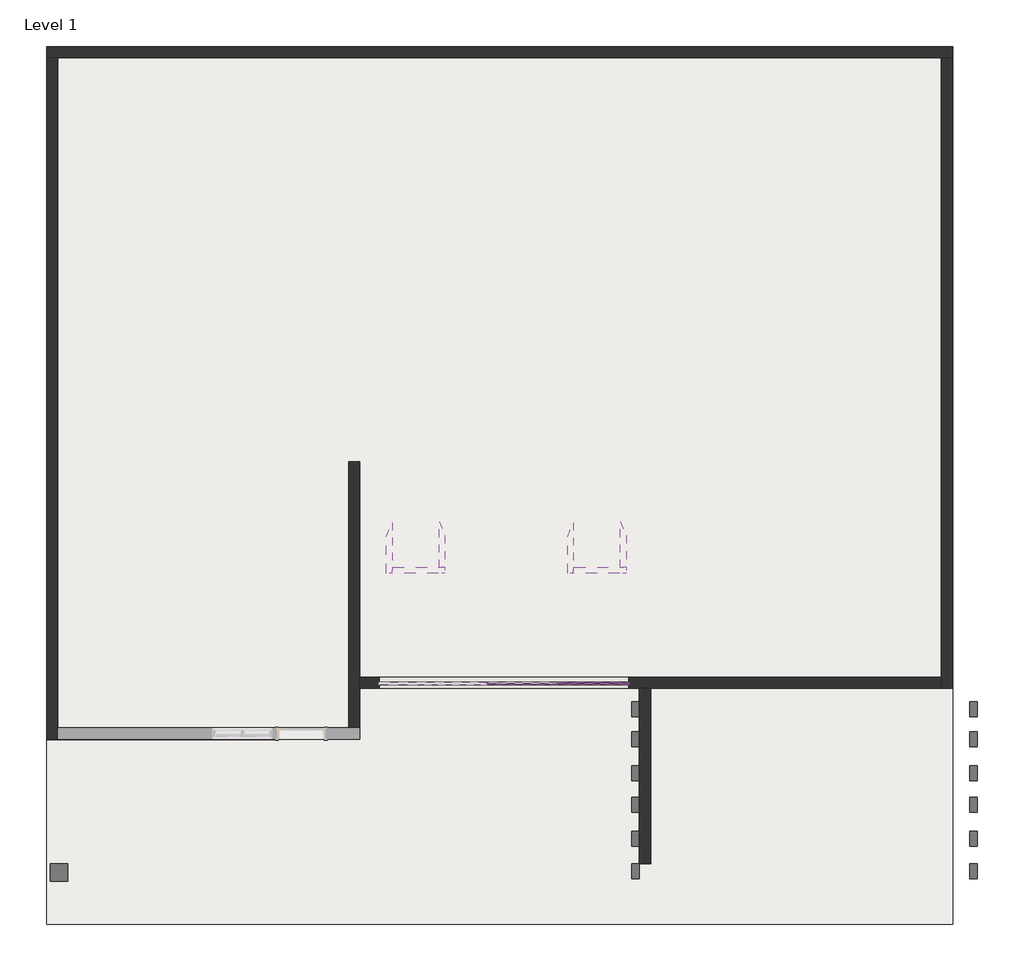
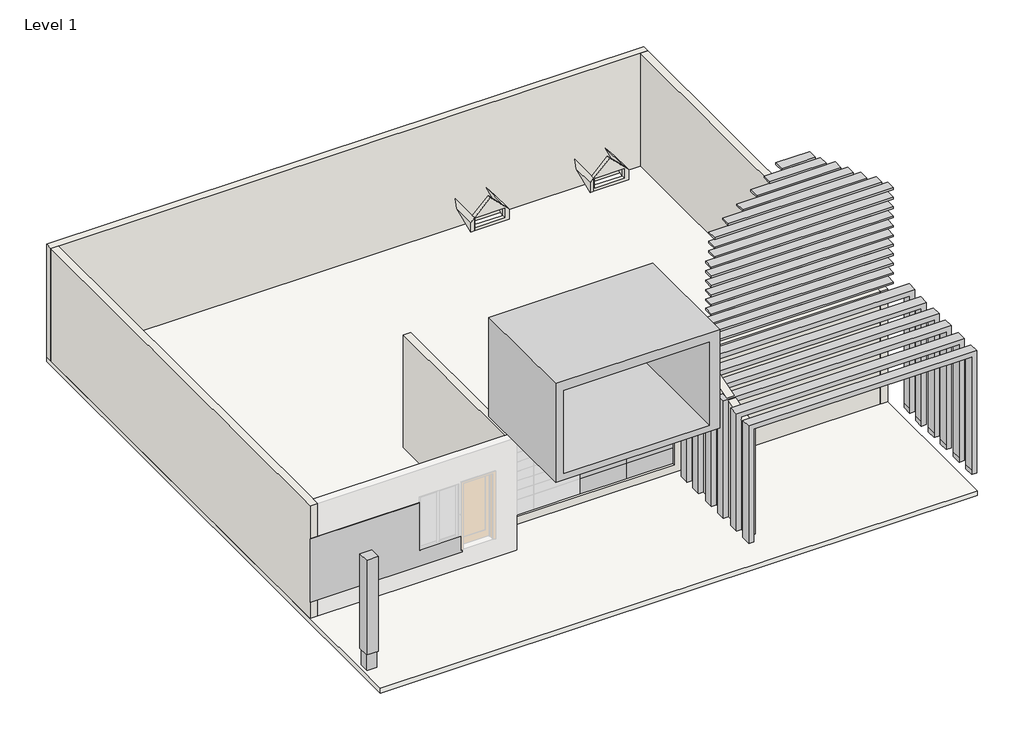
# One storey, part 2 of 2: 33 members, 16 plates, 12 walls, 1 proxy, 1 slab.
"""IFC4 building model written with IfcOpenShell, lengths in millimetres."""

from ifc_helpers import new_model, si_unit, frame, origin, place, context, project, spatial, polyline, outline, extrude, faceted_brep, transform, mapped, element, save
from components import generic_models_2_generic_models_2_f6a97bfe, member_408d7f8b, member_84ecdb2b, member_5ac041f4, member_20a2445f, member_63f4cac5, member_d020295e, member_b7a731ef, member_839e3c67, member_84e80635, system_panel_glazed_d4e05dc3, system_panel_glazed_d663d970, system_panel_glazed_cac74210

model = new_model("IFC4")

# Units and contexts
model_context = context("Model", 3, world=origin())
ifc_project = project(units=[si_unit("LENGTHUNIT", "METRE", prefix="MILLI")], contexts=[model_context])

# Site, building, storey
site = spatial("IfcSite", under=ifc_project)
building = spatial("IfcBuilding", under=site)
storey = spatial("IfcBuildingStorey", under=building, Name="Level 1", Elevation=0.0)

# Proxy
placement = place(None, origin())
generic_models_2_generic_models_2_shape = generic_models_2_generic_models_2_f6a97bfe(model_context)
element("IfcBuildingElementProxy", 1, Name="Generic Models 2 : Generic Models 2", ObjectType="Generic Models 2 : Generic Models 2", at=placement, inside=storey, context=model_context, shape_type="MappedRepresentation", body=[
    mapped(generic_models_2_generic_models_2_shape, transform((0.0, 0.0, 0.0), x_axis=(1.0, 0.0, 0.0), y_axis=(0.0, 1.0, 0.0), z_axis=(0.0, 0.0, 1.0))),
])

# Members
member_shape = member_408d7f8b(model_context)
element("IfcMember", 2, ObjectType="Rectangular Mullion : 1\" Square", at=placement, inside=storey, context=model_context, shape_type="MappedRepresentation", body=[
    mapped(member_shape, transform((-1613.8294011, -1238.9111529, 247.9343309), x_axis=(0.0, 0.0, -1.0), y_axis=(0.0, 1.0, 0.0), z_axis=(1.0, 0.0, 0.0))),
])
member_2_shape = member_84ecdb2b(model_context)
element("IfcMember", 3, ObjectType="Rectangular Mullion : 1\" Square", at=placement, inside=storey, context=model_context, shape_type="MappedRepresentation", body=[
    mapped(member_2_shape, transform((-2998.1294011, -1238.9111529, 2572.3741932), x_axis=(0.0, 0.0, 1.0), y_axis=(0.0, 1.0, 0.0), z_axis=(-1.0, 0.0, 0.0))),
])
element("IfcMember", 4, ObjectType="Rectangular Mullion : 1\" Square", at=placement, inside=storey, context=model_context, shape_type="MappedRepresentation", body=[
    mapped(member_2_shape, transform((-2998.1294011, -1238.9111529, 2267.5741932), x_axis=(0.0, 0.0, 1.0), y_axis=(0.0, 1.0, 0.0), z_axis=(-1.0, 0.0, 0.0))),
])
element("IfcMember", 5, ObjectType="Rectangular Mullion : 1\" Square", at=placement, inside=storey, context=model_context, shape_type="MappedRepresentation", body=[
    mapped(member_2_shape, transform((-2998.1294011, -1238.9111529, 1962.7741932), x_axis=(0.0, 0.0, 1.0), y_axis=(0.0, 1.0, 0.0), z_axis=(-1.0, 0.0, 0.0))),
])
element("IfcMember", 6, ObjectType="Rectangular Mullion : 1\" Square", at=placement, inside=storey, context=model_context, shape_type="MappedRepresentation", body=[
    mapped(member_2_shape, transform((-2998.1294011, -1238.9111529, 1353.1741932), x_axis=(0.0, 0.0, 1.0), y_axis=(0.0, 1.0, 0.0), z_axis=(-1.0, 0.0, 0.0))),
])
element("IfcMember", 7, ObjectType="Rectangular Mullion : 1\" Square", at=placement, inside=storey, context=model_context, shape_type="MappedRepresentation", body=[
    mapped(member_2_shape, transform((-2998.1294011, -1238.9111529, 1657.9741932), x_axis=(0.0, 0.0, 1.0), y_axis=(0.0, 1.0, 0.0), z_axis=(-1.0, 0.0, 0.0))),
])
element("IfcMember", 8, ObjectType="Rectangular Mullion : 1\" Square", at=placement, inside=storey, context=model_context, shape_type="MappedRepresentation", body=[
    mapped(member_2_shape, transform((-2998.1294011, -1238.9111529, 1048.3741932), x_axis=(0.0, 0.0, 1.0), y_axis=(0.0, 1.0, 0.0), z_axis=(-1.0, 0.0, 0.0))),
])
element("IfcMember", 9, ObjectType="Rectangular Mullion : 1\" Square", at=placement, inside=storey, context=model_context, shape_type="MappedRepresentation", body=[
    mapped(member_2_shape, transform((-2998.1294011, -1238.9111529, 743.5741932), x_axis=(0.0, 0.0, 1.0), y_axis=(0.0, 1.0, 0.0), z_axis=(-1.0, 0.0, 0.0))),
])
member_3_shape = member_5ac041f4(model_context)
element("IfcMember", 10, ObjectType="Rectangular Mullion : 1\" Square", at=placement, inside=storey, context=model_context, shape_type="MappedRepresentation", body=[
    mapped(member_3_shape, transform((-3010.8294011, -1238.9111529, 247.9343309), x_axis=(-1.0, 0.0, 0.0), y_axis=(0.0, 1.0, 0.0), z_axis=(0.0, 0.0, -1.0))),
])
member_4_shape = member_20a2445f(model_context)
element("IfcMember", 11, ObjectType="Rectangular Mullion : 1\" Square", at=placement, inside=storey, context=model_context, shape_type="MappedRepresentation", body=[
    mapped(member_4_shape, transform((-3023.5294011, -1238.9111529, 247.9343309), x_axis=(0.0, 0.0, -1.0), y_axis=(0.0, 1.0, 0.0), z_axis=(1.0, 0.0, 0.0))),
])
element("IfcMember", 12, ObjectType="Rectangular Mullion : 1\" Square", at=placement, inside=storey, context=model_context, shape_type="MappedRepresentation", body=[
    mapped(member_shape, transform((-2998.1294011, -1238.9111529, 2823.4928635), x_axis=(0.0, 0.0, 1.0), y_axis=(0.0, 1.0, 0.0), z_axis=(-1.0, 0.0, 0.0))),
])
member_5_shape = member_63f4cac5(model_context)
element("IfcMember", 13, ObjectType="Rectangular Mullion : 1\" Square", at=placement, inside=storey, context=model_context, shape_type="MappedRepresentation", body=[
    mapped(member_5_shape, transform((-4433.2294011, -1238.9111529, 2572.3741932), x_axis=(-1.0, 0.0, 0.0), y_axis=(0.0, 1.0, 0.0), z_axis=(0.0, 0.0, -1.0))),
])
element("IfcMember", 14, ObjectType="Rectangular Mullion : 1\" Square", at=placement, inside=storey, context=model_context, shape_type="MappedRepresentation", body=[
    mapped(member_5_shape, transform((-3010.8294011, -1238.9111529, 2572.3741932), x_axis=(-1.0, 0.0, 0.0), y_axis=(0.0, 1.0, 0.0), z_axis=(0.0, 0.0, -1.0))),
])
member_6_shape = member_d020295e(model_context)
element("IfcMember", 15, ObjectType="Rectangular Mullion : 1\" Square", at=placement, inside=storey, context=model_context, shape_type="MappedRepresentation", body=[
    mapped(member_6_shape, transform((-4433.2294011, -1238.9111529, 2267.5741932), x_axis=(-1.0, 0.0, 0.0), y_axis=(0.0, 1.0, 0.0), z_axis=(0.0, 0.0, -1.0))),
])
element("IfcMember", 16, ObjectType="Rectangular Mullion : 1\" Square", at=placement, inside=storey, context=model_context, shape_type="MappedRepresentation", body=[
    mapped(member_6_shape, transform((-4433.2294011, -1238.9111529, 1962.7741932), x_axis=(-1.0, 0.0, 0.0), y_axis=(0.0, 1.0, 0.0), z_axis=(0.0, 0.0, -1.0))),
])
element("IfcMember", 17, ObjectType="Rectangular Mullion : 1\" Square", at=placement, inside=storey, context=model_context, shape_type="MappedRepresentation", body=[
    mapped(member_6_shape, transform((-4433.2294011, -1238.9111529, 1353.1741932), x_axis=(-1.0, 0.0, 0.0), y_axis=(0.0, 1.0, 0.0), z_axis=(0.0, 0.0, -1.0))),
])
element("IfcMember", 18, ObjectType="Rectangular Mullion : 1\" Square", at=placement, inside=storey, context=model_context, shape_type="MappedRepresentation", body=[
    mapped(member_6_shape, transform((-4433.2294011, -1238.9111529, 1657.9741932), x_axis=(-1.0, 0.0, 0.0), y_axis=(0.0, 1.0, 0.0), z_axis=(0.0, 0.0, -1.0))),
])
element("IfcMember", 19, ObjectType="Rectangular Mullion : 1\" Square", at=placement, inside=storey, context=model_context, shape_type="MappedRepresentation", body=[
    mapped(member_6_shape, transform((-4433.2294011, -1238.9111529, 1048.3741932), x_axis=(-1.0, 0.0, 0.0), y_axis=(0.0, 1.0, 0.0), z_axis=(0.0, 0.0, -1.0))),
])
element("IfcMember", 20, ObjectType="Rectangular Mullion : 1\" Square", at=placement, inside=storey, context=model_context, shape_type="MappedRepresentation", body=[
    mapped(member_6_shape, transform((-4433.2294011, -1238.9111529, 743.5741932), x_axis=(-1.0, 0.0, 0.0), y_axis=(0.0, 1.0, 0.0), z_axis=(0.0, 0.0, -1.0))),
])
element("IfcMember", 21, ObjectType="Rectangular Mullion : 1\" Square", at=placement, inside=storey, context=model_context, shape_type="MappedRepresentation", body=[
    mapped(member_6_shape, transform((-3010.8294011, -1238.9111529, 2267.5741932), x_axis=(-1.0, 0.0, 0.0), y_axis=(0.0, 1.0, 0.0), z_axis=(0.0, 0.0, -1.0))),
])
element("IfcMember", 22, ObjectType="Rectangular Mullion : 1\" Square", at=placement, inside=storey, context=model_context, shape_type="MappedRepresentation", body=[
    mapped(member_6_shape, transform((-3010.8294011, -1238.9111529, 1962.7741932), x_axis=(-1.0, 0.0, 0.0), y_axis=(0.0, 1.0, 0.0), z_axis=(0.0, 0.0, -1.0))),
])
element("IfcMember", 23, ObjectType="Rectangular Mullion : 1\" Square", at=placement, inside=storey, context=model_context, shape_type="MappedRepresentation", body=[
    mapped(member_6_shape, transform((-3010.8294011, -1238.9111529, 1353.1741932), x_axis=(-1.0, 0.0, 0.0), y_axis=(0.0, 1.0, 0.0), z_axis=(0.0, 0.0, -1.0))),
])
element("IfcMember", 24, ObjectType="Rectangular Mullion : 1\" Square", at=placement, inside=storey, context=model_context, shape_type="MappedRepresentation", body=[
    mapped(member_6_shape, transform((-3010.8294011, -1238.9111529, 1657.9741932), x_axis=(-1.0, 0.0, 0.0), y_axis=(0.0, 1.0, 0.0), z_axis=(0.0, 0.0, -1.0))),
])
element("IfcMember", 25, ObjectType="Rectangular Mullion : 1\" Square", at=placement, inside=storey, context=model_context, shape_type="MappedRepresentation", body=[
    mapped(member_6_shape, transform((-3010.8294011, -1238.9111529, 1048.3741932), x_axis=(-1.0, 0.0, 0.0), y_axis=(0.0, 1.0, 0.0), z_axis=(0.0, 0.0, -1.0))),
])
element("IfcMember", 26, ObjectType="Rectangular Mullion : 1\" Square", at=placement, inside=storey, context=model_context, shape_type="MappedRepresentation", body=[
    mapped(member_6_shape, transform((-3010.8294011, -1238.9111529, 743.5741932), x_axis=(-1.0, 0.0, 0.0), y_axis=(0.0, 1.0, 0.0), z_axis=(0.0, 0.0, -1.0))),
])
member_7_shape = member_b7a731ef(model_context)
element("IfcMember", 27, ObjectType="Rectangular Mullion : 1\" Square", at=placement, inside=storey, context=model_context, shape_type="MappedRepresentation", body=[
    mapped(member_7_shape, transform((-1588.4294011, -1238.9111529, 2823.4928635), x_axis=(1.0, 0.0, 0.0), y_axis=(0.0, 1.0, 0.0), z_axis=(0.0, 0.0, 1.0))),
])
member_8_shape = member_839e3c67(model_context)
element("IfcMember", 28, ObjectType="Rectangular Mullion : 1\" Square", at=placement, inside=storey, context=model_context, shape_type="MappedRepresentation", body=[
    mapped(member_8_shape, transform((-1588.4294011, -1238.9111529, 2572.3741932), x_axis=(1.0, 0.0, 0.0), y_axis=(0.0, 1.0, 0.0), z_axis=(0.0, 0.0, 1.0))),
])
element("IfcMember", 29, ObjectType="Rectangular Mullion : 1\" Square", at=placement, inside=storey, context=model_context, shape_type="MappedRepresentation", body=[
    mapped(member_8_shape, transform((-1588.4294011, -1238.9111529, 2267.5741932), x_axis=(1.0, 0.0, 0.0), y_axis=(0.0, 1.0, 0.0), z_axis=(0.0, 0.0, 1.0))),
])
element("IfcMember", 30, ObjectType="Rectangular Mullion : 1\" Square", at=placement, inside=storey, context=model_context, shape_type="MappedRepresentation", body=[
    mapped(member_8_shape, transform((-1588.4294011, -1238.9111529, 1962.7741932), x_axis=(1.0, 0.0, 0.0), y_axis=(0.0, 1.0, 0.0), z_axis=(0.0, 0.0, 1.0))),
])
element("IfcMember", 31, ObjectType="Rectangular Mullion : 1\" Square", at=placement, inside=storey, context=model_context, shape_type="MappedRepresentation", body=[
    mapped(member_8_shape, transform((-1588.4294011, -1238.9111529, 1353.1741932), x_axis=(1.0, 0.0, 0.0), y_axis=(0.0, 1.0, 0.0), z_axis=(0.0, 0.0, 1.0))),
])
element("IfcMember", 32, ObjectType="Rectangular Mullion : 1\" Square", at=placement, inside=storey, context=model_context, shape_type="MappedRepresentation", body=[
    mapped(member_8_shape, transform((-1588.4294011, -1238.9111529, 1657.9741932), x_axis=(1.0, 0.0, 0.0), y_axis=(0.0, 1.0, 0.0), z_axis=(0.0, 0.0, 1.0))),
])
element("IfcMember", 33, ObjectType="Rectangular Mullion : 1\" Square", at=placement, inside=storey, context=model_context, shape_type="MappedRepresentation", body=[
    mapped(member_8_shape, transform((-1588.4294011, -1238.9111529, 1048.3741932), x_axis=(1.0, 0.0, 0.0), y_axis=(0.0, 1.0, 0.0), z_axis=(0.0, 0.0, 1.0))),
])
member_9_shape = member_84e80635(model_context)
element("IfcMember", 34, ObjectType="Rectangular Mullion : 1\" Square", at=placement, inside=storey, context=model_context, shape_type="MappedRepresentation", body=[
    mapped(member_9_shape, transform((-1588.4294011, -1238.9111529, 743.5741932), x_axis=(1.0, 0.0, 0.0), y_axis=(0.0, 1.0, 0.0), z_axis=(0.0, 0.0, 1.0))),
])

# Plates
system_panel_glazed_shape = system_panel_glazed_d4e05dc3(model_context)
element("IfcPlate", 35, ObjectType="System Panel : Glazed", at=placement, inside=storey, context=model_context, shape_type="MappedRepresentation", body=[
    mapped(system_panel_glazed_shape, transform((-2299.6294011, -1238.9111529, 247.9343309), x_axis=(-1.0, 0.0, 0.0), y_axis=(0.0, -1.0, 0.0), z_axis=(0.0, 0.0, 1.0))),
])
element("IfcPlate", 36, ObjectType="System Panel : Glazed", at=placement, inside=storey, context=model_context, shape_type="MappedRepresentation", body=[
    mapped(system_panel_glazed_shape, transform((-3722.0294011, -1238.9111529, 247.9343309), x_axis=(-1.0, 0.0, 0.0), y_axis=(0.0, -1.0, 0.0), z_axis=(0.0, 0.0, 1.0))),
])
system_panel_glazed_2_shape = system_panel_glazed_d663d970(model_context)
element("IfcPlate", 37, ObjectType="System Panel : Glazed", at=placement, inside=storey, context=model_context, shape_type="MappedRepresentation", body=[
    mapped(system_panel_glazed_2_shape, transform((-2299.6294011, -1238.9111529, 2267.5741932), x_axis=(-1.0, 0.0, 0.0), y_axis=(0.0, -1.0, 0.0), z_axis=(0.0, 0.0, 1.0))),
])
element("IfcPlate", 38, ObjectType="System Panel : Glazed", at=placement, inside=storey, context=model_context, shape_type="MappedRepresentation", body=[
    mapped(system_panel_glazed_2_shape, transform((-2299.6294011, -1238.9111529, 1962.7741932), x_axis=(-1.0, 0.0, 0.0), y_axis=(0.0, -1.0, 0.0), z_axis=(0.0, 0.0, 1.0))),
])
element("IfcPlate", 39, ObjectType="System Panel : Glazed", at=placement, inside=storey, context=model_context, shape_type="MappedRepresentation", body=[
    mapped(system_panel_glazed_2_shape, transform((-2299.6294011, -1238.9111529, 1353.1741932), x_axis=(-1.0, 0.0, 0.0), y_axis=(0.0, -1.0, 0.0), z_axis=(0.0, 0.0, 1.0))),
])
element("IfcPlate", 40, ObjectType="System Panel : Glazed", at=placement, inside=storey, context=model_context, shape_type="MappedRepresentation", body=[
    mapped(system_panel_glazed_2_shape, transform((-2299.6294011, -1238.9111529, 1657.9741932), x_axis=(-1.0, 0.0, 0.0), y_axis=(0.0, -1.0, 0.0), z_axis=(0.0, 0.0, 1.0))),
])
element("IfcPlate", 41, ObjectType="System Panel : Glazed", at=placement, inside=storey, context=model_context, shape_type="MappedRepresentation", body=[
    mapped(system_panel_glazed_2_shape, transform((-2299.6294011, -1238.9111529, 1048.3741932), x_axis=(-1.0, 0.0, 0.0), y_axis=(0.0, -1.0, 0.0), z_axis=(0.0, 0.0, 1.0))),
])
element("IfcPlate", 42, ObjectType="System Panel : Glazed", at=placement, inside=storey, context=model_context, shape_type="MappedRepresentation", body=[
    mapped(system_panel_glazed_2_shape, transform((-2299.6294011, -1238.9111529, 743.5741932), x_axis=(-1.0, 0.0, 0.0), y_axis=(0.0, -1.0, 0.0), z_axis=(0.0, 0.0, 1.0))),
])
element("IfcPlate", 43, ObjectType="System Panel : Glazed", at=placement, inside=storey, context=model_context, shape_type="MappedRepresentation", body=[
    mapped(system_panel_glazed_2_shape, transform((-3722.0294011, -1238.9111529, 743.5741932), x_axis=(-1.0, 0.0, 0.0), y_axis=(0.0, -1.0, 0.0), z_axis=(0.0, 0.0, 1.0))),
])
element("IfcPlate", 44, ObjectType="System Panel : Glazed", at=placement, inside=storey, context=model_context, shape_type="MappedRepresentation", body=[
    mapped(system_panel_glazed_2_shape, transform((-3722.0294011, -1238.9111529, 1048.3741932), x_axis=(-1.0, 0.0, 0.0), y_axis=(0.0, -1.0, 0.0), z_axis=(0.0, 0.0, 1.0))),
])
element("IfcPlate", 45, ObjectType="System Panel : Glazed", at=placement, inside=storey, context=model_context, shape_type="MappedRepresentation", body=[
    mapped(system_panel_glazed_2_shape, transform((-3722.0294011, -1238.9111529, 1353.1741932), x_axis=(-1.0, 0.0, 0.0), y_axis=(0.0, -1.0, 0.0), z_axis=(0.0, 0.0, 1.0))),
])
element("IfcPlate", 46, ObjectType="System Panel : Glazed", at=placement, inside=storey, context=model_context, shape_type="MappedRepresentation", body=[
    mapped(system_panel_glazed_2_shape, transform((-3722.0294011, -1238.9111529, 1657.9741932), x_axis=(-1.0, 0.0, 0.0), y_axis=(0.0, -1.0, 0.0), z_axis=(0.0, 0.0, 1.0))),
])
element("IfcPlate", 47, ObjectType="System Panel : Glazed", at=placement, inside=storey, context=model_context, shape_type="MappedRepresentation", body=[
    mapped(system_panel_glazed_2_shape, transform((-3722.0294011, -1238.9111529, 1962.7741932), x_axis=(-1.0, 0.0, 0.0), y_axis=(0.0, -1.0, 0.0), z_axis=(0.0, 0.0, 1.0))),
])
element("IfcPlate", 48, ObjectType="System Panel : Glazed", at=placement, inside=storey, context=model_context, shape_type="MappedRepresentation", body=[
    mapped(system_panel_glazed_2_shape, transform((-3722.0294011, -1238.9111529, 2267.5741932), x_axis=(-1.0, 0.0, 0.0), y_axis=(0.0, -1.0, 0.0), z_axis=(0.0, 0.0, 1.0))),
])
system_panel_glazed_3_shape = system_panel_glazed_cac74210(model_context)
element("IfcPlate", 49, ObjectType="System Panel : Glazed", at=placement, inside=storey, context=model_context, shape_type="MappedRepresentation", body=[
    mapped(system_panel_glazed_3_shape, transform((-2299.6294011, -1238.9111529, 2572.3741932), x_axis=(-1.0, 0.0, 0.0), y_axis=(0.0, -1.0, 0.0), z_axis=(0.0, 0.0, 1.0))),
])
element("IfcPlate", 50, ObjectType="System Panel : Glazed", at=placement, inside=storey, context=model_context, shape_type="MappedRepresentation", body=[
    mapped(system_panel_glazed_3_shape, transform((-3722.0294011, -1238.9111529, 2572.3741932), x_axis=(-1.0, 0.0, 0.0), y_axis=(0.0, -1.0, 0.0), z_axis=(0.0, 0.0, 1.0))),
])

# Slab
element("IfcSlab", 51, ObjectType="6\" floor", at=placement, inside=storey, context=model_context, shape_type="SweptSolid", body=[
    extrude(outline(polyline([(4952.0705989, 11600.7888471), (4952.0705989, -6115.7111529), (-13335.9294011, -6115.7111529), (-13335.9294011, 11600.7888471), (4952.0705989, 11600.7888471)])), frame((0.0, 0.0, -152.4), z_axis=(0.0, 0.0, 1.0), x_axis=(1.0, 0.0, 0.0)), (0.0, 0.0, 1.0), 152.4),
])

# Walls
element("IfcWall", 52, ObjectType="4.5\" wall", at=placement, inside=storey, context=model_context, shape_type="Brep", body=[
    faceted_brep([(-6362.1186248, 1982.9905218, 8519.2266783), (-6362.1186248, 1085.1888471, 8519.2266783), (-6362.1186248, 970.8888471, 8519.2266783), (-6362.1186248, 970.8888471, 8096.1555912), (-6362.1186248, 1085.1888471, 8143.9344127), (-6476.4186248, 970.8888471, 8096.1555912), (-6476.4186248, 970.8888471, 8404.9266783), (-6476.4186248, 1709.5536812, 8404.9266783)], [[[0, 1, 2, 3, 4]], [[5, 6, 7]], [[2, 6, 5, 3]], [[6, 2, 1, 0, 7]], [[0, 4, 3, 5, 7]]]),
])
element("IfcWall", 53, ObjectType="4.5\" wall", at=placement, inside=storey, context=model_context, shape_type="Brep", body=[
    faceted_brep([(-5295.3186248, 1085.1888471, 8414.6051258), (-5295.3186248, 1085.1888471, 8143.9344127), (-5409.6186248, 1085.1888471, 8143.9344127), (-6362.1186248, 1085.1888471, 8143.9344127), (-6362.1186248, 1085.1888471, 8519.2266783), (-5881.0294011, 1085.1888471, 9000.3159021), (-5409.6186248, 1085.1888471, 8528.9051258), (-5428.6686248, 1085.1888471, 8192.8954339), (-5428.6686248, 1085.1888471, 8497.6954339), (-6343.0686248, 1085.1888471, 8497.6954339), (-6343.0686248, 1085.1888471, 8192.8954339), (-5295.3186248, 970.8888471, 8096.1555912), (-5295.3186248, 970.8888471, 8414.6051258), (-5881.0294011, 970.8888471, 9000.3159021), (-6362.1186248, 970.8888471, 8519.2266783), (-6362.1186248, 970.8888471, 8096.1555912), (-5428.6686248, 970.8888471, 8497.6954339), (-5428.6686248, 970.8888471, 8192.8954339), (-6343.0686248, 970.8888471, 8192.8954339), (-6343.0686248, 970.8888471, 8497.6954339)], [[[0, 1, 2, 3, 4, 5, 6], [7, 8, 9, 10]], [[11, 12, 13, 14, 15], [16, 17, 18, 19]], [[1, 0, 12, 11]], [[4, 3, 15, 14]], [[12, 0, 6, 5, 13]], [[4, 14, 13, 5]], [[3, 2, 1, 11, 15]], [[16, 8, 7, 17]], [[17, 7, 10, 18]], [[18, 10, 9, 19]], [[8, 16, 19, 9]]]),
])
element("IfcWall", 54, ObjectType="4.5\" wall", at=placement, inside=storey, context=model_context, shape_type="Brep", body=[
    faceted_brep([(-5409.6186248, 1085.1888471, 8143.9344127), (-5409.6186248, 1085.1888471, 8528.9051258), (-5409.6186248, 2006.1440134, 8528.9051258), (-5295.3186248, 1732.7071728, 8414.6051258), (-5295.3186248, 1085.1888471, 8414.6051258), (-5295.3186248, 1085.1888471, 8143.9344127)], [[[0, 1, 2]], [[3, 4, 5]], [[4, 1, 0, 5]], [[1, 4, 3, 2]], [[0, 2, 3, 5]]]),
])
element("IfcWall", 55, ObjectType="4.5\" wall", at=placement, inside=storey, context=model_context, shape_type="Brep", body=[
    faceted_brep([(-2704.5186248, 1982.9905218, 8519.2266783), (-2704.5186248, 1085.1888471, 8519.2266783), (-2704.5186248, 970.8888471, 8519.2266783), (-2704.5186248, 970.8888471, 8096.1555912), (-2704.5186248, 1085.1888471, 8143.9344127), (-2818.8186248, 970.8888471, 8096.1555912), (-2818.8186248, 970.8888471, 8404.9266783), (-2818.8186248, 1709.5536812, 8404.9266783)], [[[0, 1, 2, 3, 4]], [[5, 6, 7]], [[2, 6, 5, 3]], [[6, 2, 1, 0, 7]], [[0, 4, 3, 5, 7]]]),
])
element("IfcWall", 56, ObjectType="4.5\" wall", at=placement, inside=storey, context=model_context, shape_type="Brep", body=[
    faceted_brep([(-1637.7186248, 1085.1888471, 8414.6051258), (-1637.7186248, 1085.1888471, 8143.9344127), (-1752.0186248, 1085.1888471, 8143.9344127), (-2704.5186248, 1085.1888471, 8143.9344127), (-2704.5186248, 1085.1888471, 8519.2266783), (-2223.4294011, 1085.1888471, 9000.3159021), (-1752.0186248, 1085.1888471, 8528.9051258), (-1771.0686248, 1085.1888471, 8192.8954339), (-1771.0686248, 1085.1888471, 8497.6954339), (-2685.4686248, 1085.1888471, 8497.6954339), (-2685.4686248, 1085.1888471, 8192.8954339), (-1637.7186248, 970.8888471, 8096.1555912), (-1637.7186248, 970.8888471, 8414.6051258), (-2223.4294011, 970.8888471, 9000.3159021), (-2704.5186248, 970.8888471, 8519.2266783), (-2704.5186248, 970.8888471, 8096.1555912), (-1771.0686248, 970.8888471, 8497.6954339), (-1771.0686248, 970.8888471, 8192.8954339), (-2685.4686248, 970.8888471, 8192.8954339), (-2685.4686248, 970.8888471, 8497.6954339)], [[[0, 1, 2, 3, 4, 5, 6], [7, 8, 9, 10]], [[11, 12, 13, 14, 15], [16, 17, 18, 19]], [[1, 0, 12, 11]], [[4, 3, 15, 14]], [[12, 0, 6, 5, 13]], [[4, 14, 13, 5]], [[3, 2, 1, 11, 15]], [[16, 8, 7, 17]], [[17, 7, 10, 18]], [[18, 10, 9, 19]], [[8, 16, 19, 9]]]),
])
element("IfcWall", 57, ObjectType="4.5\" wall", at=placement, inside=storey, context=model_context, shape_type="Brep", body=[
    faceted_brep([(-1752.0186248, 1085.1888471, 8143.9344127), (-1752.0186248, 1085.1888471, 8528.9051258), (-1752.0186248, 2006.1440134, 8528.9051258), (-1637.7186248, 1732.7071728, 8414.6051258), (-1637.7186248, 1085.1888471, 8414.6051258), (-1637.7186248, 1085.1888471, 8143.9344127)], [[[0, 1, 2]], [[3, 4, 5]], [[4, 1, 0, 5]], [[1, 4, 3, 2]], [[0, 2, 3, 5]]]),
])
element("IfcWall", 58, ObjectType="9\" wall", at=placement, inside=storey, context=model_context, shape_type="Brep", body=[
    faceted_brep([(-13335.9294011, 11372.1888471, 0.0), (-13107.3294011, 11372.1888471, 0.0), (4723.4705989, 11372.1888471, 0.0), (4952.0705989, 11372.1888471, 0.0), (4952.0705989, 11372.1888471, 3657.6), (4723.4705989, 11372.1888471, 3657.6), (-13107.3294011, 11372.1888471, 3657.6), (-13335.9294011, 11372.1888471, 3657.6), (-13335.9294011, 11600.7888471, 0.0), (-13335.9294011, 11600.7888471, 3657.6), (4952.0705989, 11600.7888471, 3657.6), (4952.0705989, 11600.7888471, 0.0)], [[[0, 1, 2, 3, 4, 5, 6, 7]], [[8, 9, 10, 11]], [[3, 2, 1, 0, 8, 11]], [[7, 6, 5, 4, 10, 9]], [[4, 3, 11, 10]], [[0, 7, 9, 8]]]),
])
element("IfcWall", 59, ObjectType="9\" wall", at=placement, inside=storey, context=model_context, shape_type="Brep", body=[
    faceted_brep([(4723.4705989, 11372.1888471, 0.0), (4723.4705989, -1124.6111529, 0.0), (4723.4705989, -1353.2111529, 0.0), (4723.4705989, -1353.2111529, 3657.6), (4723.4705989, -1124.6111529, 3657.6), (4723.4705989, 11372.1888471, 3657.6), (4952.0705989, 11372.1888471, 0.0), (4952.0705989, 11372.1888471, 3657.6), (4952.0705989, -1353.2111529, 3657.6), (4952.0705989, -1353.2111529, 0.0)], [[[0, 1, 2, 3, 4, 5]], [[6, 7, 8, 9]], [[2, 1, 0, 6, 9]], [[5, 4, 3, 8, 7]], [[0, 5, 7, 6]], [[3, 2, 9, 8]]]),
])
element("IfcWall", 60, ObjectType="9\" wall", at=placement, inside=storey, context=model_context, shape_type="Brep", body=[
    faceted_brep([(4723.4705989, -1124.6111529, 0.0), (-7011.3294011, -1124.6111529, 0.0), (-7011.3294011, -1124.6111529, 3657.6), (4723.4705989, -1124.6111529, 3657.6), (-1588.4294011, -1124.6111529, 247.9343309), (-1588.4294011, -1124.6111529, 2823.4928635), (-6617.6294011, -1124.6111529, 2823.4928635), (-6617.6294011, -1124.6111529, 247.9343309), (-7011.3294011, -1353.2111529, 0.0), (-1372.5294011, -1353.2111529, 0.0), (-1143.9294011, -1353.2111529, 0.0), (4723.4705989, -1353.2111529, 0.0), (4723.4705989, -1353.2111529, 3657.6), (-7011.3294011, -1353.2111529, 3657.6), (-1588.4294011, -1353.2111529, 2823.4928635), (-1588.4294011, -1353.2111529, 247.9343309), (-6617.6294011, -1353.2111529, 247.9343309), (-6617.6294011, -1353.2111529, 2823.4928635)], [[[0, 1, 2, 3], [4, 5, 6, 7]], [[8, 9, 10, 11, 12, 13], [14, 15, 16, 17]], [[1, 0, 11, 10, 9, 8]], [[3, 2, 13, 12]], [[0, 3, 12, 11]], [[2, 1, 8, 13]], [[4, 15, 14, 5]], [[5, 14, 17, 6]], [[6, 17, 16, 7]], [[15, 4, 7, 16]]]),
])
element("IfcWall", 61, ObjectType="9\" wall", at=placement, inside=storey, context=model_context, shape_type="SweptSolid", body=[
    extrude(outline(polyline([(-1353.2111529, 0.0), (-4896.5111529, 0.0), (-4896.5111529, 3470.5559336), (-1353.2111529, 4553.8514573), (-1353.2111529, 0.0)])), frame((-1372.5294011, 0.0, 0.0), z_axis=(1.0, 0.0, 0.0), x_axis=(0.0, 1.0, 0.0)), (0.0, 0.0, 1.0), 228.6),
])
element("IfcWall", 62, ObjectType="9\" wall", at=placement, inside=storey, context=model_context, shape_type="Brep", body=[
    faceted_brep([(-13107.3294011, -2381.9111529, 0.0), (-13107.3294011, -2153.3111529, 0.0), (-13107.3294011, 11372.1888471, 0.0), (-13107.3294011, 11372.1888471, 3657.6), (-13107.3294011, -2153.3111529, 3657.6), (-13107.3294011, -2381.9111529, 3657.6), (-13335.9294011, -2381.9111529, 0.0), (-13335.9294011, -2381.9111529, 3657.6), (-13335.9294011, 11372.1888471, 3657.6), (-13335.9294011, 11372.1888471, 0.0)], [[[0, 1, 2, 3, 4, 5]], [[6, 7, 8, 9]], [[2, 1, 0, 6, 9]], [[5, 4, 3, 8, 7]], [[3, 2, 9, 8]], [[0, 5, 7, 6]]]),
])
element("IfcWall", 63, ObjectType="9\" wall", at=placement, inside=storey, context=model_context, shape_type="Brep", body=[
    faceted_brep([(-7011.3294011, -2153.3111529, 0.0), (-7011.3294011, -1353.2111529, 0.0), (-7011.3294011, -1124.6111529, 0.0), (-7011.3294011, 3218.7888471, 0.0), (-7011.3294011, 3218.7888471, 3657.6), (-7011.3294011, -1124.6111529, 3657.6), (-7011.3294011, -1353.2111529, 3657.6), (-7011.3294011, -2153.3111529, 3657.6), (-7239.9294011, -2153.3111529, 0.0), (-7239.9294011, -2153.3111529, 3657.6), (-7239.9294011, 3218.7888471, 3657.6), (-7239.9294011, 3218.7888471, 0.0)], [[[0, 1, 2, 3, 4, 5, 6, 7]], [[8, 9, 10, 11]], [[3, 2, 1, 0, 8, 11]], [[4, 3, 11, 10]], [[7, 6, 5, 4, 10, 9]], [[0, 7, 9, 8]]]),
])

save(model, "model.ifc")

# Revit data of these elements
# Type "Rectangular Mullion : 1\" Square"
#   built-in parameter 1007304 = 0.0833333 (stored number, unit not read)
#   built-in parameter 1007301 = 0.0416667 (stored number, unit not read)
#   built-in parameter 1007300 = 0.0416667 (stored number, unit not read)
# Type "System Panel : Glazed"
#   Construction Type Id = "GSP4R"
#   Analytic Construction = "1/8 in Pilkington single glazing"
#   Visual Light Transmittance = 0.9
#   Solar Heat Gain Coefficient = 0.86
#   Heat Transfer Coefficient (U) = 1.18115 BTU/(h·ft²·°F)
#   Define Thermal Properties by = 1
# Type "6\" floor"
#   Assembly Code = "B1010"
#   Function = 0
#   Layers, outside or top first: 0' - 6" no material (function 1)
# Type "4.5\" wall"
#   Assembly Code = "B2010"
#   Layers, outside or top first: 0' - 4 1/2" "Gypsum Wall Board" (function 1)
# Type "9\" wall"
#   Assembly Code = "B2010"
#   Layers, outside or top first: 0' - 9" "Gypsum Wall Board" (function 1)
# Element 1 (IfcBuildingElementProxy, "Generic Models 2 : Generic Models 2")
#   Phase Created = New Construction
#   Materials on its faces: "Gypsum Wall Board", "tiles"
# Elements 2, 3, 4, 5, 6, 7, 8, 9, 10, 11, 12, 13, 14, 15, 16, 17, 18, 19, 20, 21, 22, 23, 24, 25, 26, 27, 28, 29, 30, 31, 32, 33, 34 (IfcMember, "Rectangular Mullion : 1\" Square")
#   Phase Created = New Construction
# Elements 35, 36, 37, 38, 39, 40, 41, 42, 43, 44, 45, 46, 47, 48, 49, 50 (IfcPlate, "System Panel : Glazed")
#   Phase Created = New Construction
#   Materials on its faces: "Glass"
# Element 51 (IfcSlab, "6\" floor")
#   Height Offset From Level = 0' - 0"
#   Phase Created = New Construction
#   Materials on its faces: "Default Floor"
# Elements 52, 53, 54, 55, 56, 57 (IfcWall, "4.5\" wall")
#   Top Offset = 2' - 0"
#   Base Offset = 0' - 0"
#   wall height = 14' - 0"
#   Phase Created = New Construction
#   Base Constraint = Level 1
#   Top Constraint = Level 2
#   Materials on its faces: "Gypsum Wall Board"
# Elements 58, 59, 60, 61, 62, 63 (IfcWall, "9\" wall")
#   Top Offset = 0' - 0"
#   Base Offset = 0' - 0"
#   wall height = 12' - 0"
#   Phase Created = New Construction
#   Base Constraint = Level 1
#   Top Constraint = Level 2
#   Materials on its faces: "Gypsum Wall Board"
# Materials
#   "Gypsum Wall Board": class "Generic", colour RGB 127 127 127, transparency 0, Description = "Gypsum Wall Board", Cost = 0
#   "tiles": class "Generic", colour RGB 120 120 120, transparency 0, Cost = 0
#   "Glass": class "Glass", colour RGB 0 128 192, transparency 0.75, Description = "Soda Lime Glass", Cost = 0
#   "Default Floor": colour RGB 128 128 128, transparency 0, Cost = 0
